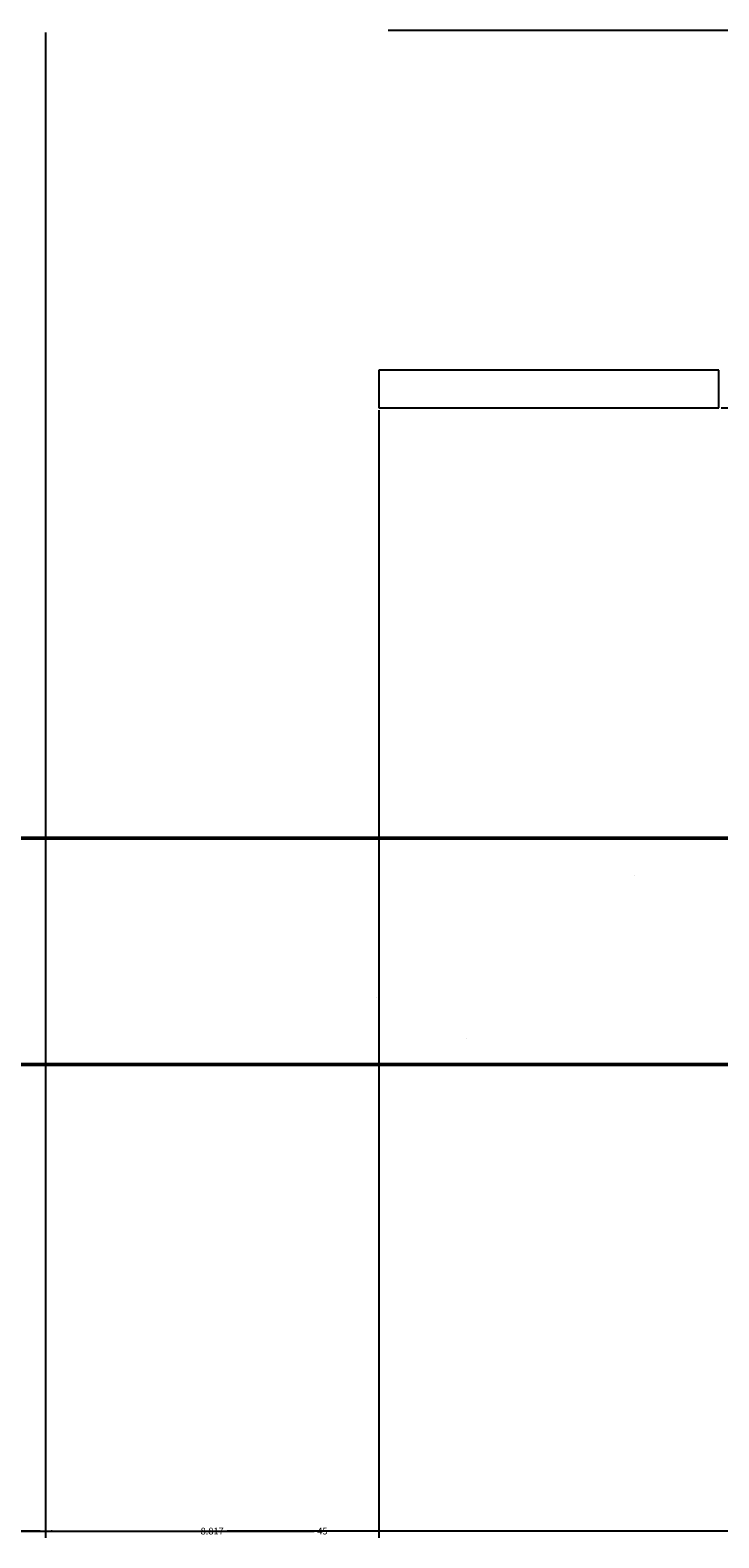
# Model space of a CAD drawing. Units: inches. Extents: x 2812 to 3051, y 1398 to 1659.
# Tile 15 of 65: x 2911 to 2929, y 1398 to 1437. Entities that reach past the tile are written whole.
import ezdxf

# ---------------------------------------------------------------- set-up
doc = ezdxf.new("R2010")
doc.units = ezdxf.units.IN
for name, color, linetype, lineweight in [('A-ANNO-DIMS', 2, 'Continuous', 18), ('S-CONC', 7, 'Continuous', 50), ('S-CONC-PATT', 8, 'Continuous', 18), ('S-STEP', 3, 'Continuous', 25)]:
    doc.layers.add(name, color=color, linetype=linetype, lineweight=lineweight)
doc.styles.get("Standard").update_dxf_attribs({"font": 'arial.ttf'})
doc.dimstyles.get("Standard").update_dxf_attribs({"dimtxt": 0.18, "dimasz": 0.18, "dimexe": 0.18, "dimexo": 0.0625, "dimgap": 0.09, "dimtad": 0, "dimtih": 1, "dimtoh": 1, "dimdec": 4, "dimzin": 0, "dimdsep": 46, "dimtxsty": 'Standard', "dimcen": 0.09, "dimadec": 0, "dimazin": 0, "dimtfac": 1, "dimtdec": 4, "dimtofl": 0, "dimtmove": 0, "dimatfit": 3, "dimfxl": 1, "dimtolj": 1, "dimtzin": 0, "dimarcsym": 0})

# ---------------------------------------------------------------- blocks, each defined once
blk = doc.blocks.new('STEP-IRON-3')
for p, q in [((9, 1), (0, 1)), ((0, 1), (0, 0)), ((9, 0), (9, 1)), ((0, 0), (4.457, 0)), ((0, 0), (9, 0)), ((0, 0), (5.792, 0))]:
    blk.add_line(p, q)
blk = doc.blocks.new('*D45')
at = {"layer": 'A-ANNO-DIMS', "color": 0, "lineweight": -2, "transparency": 16777216}
for p, q in [((2896.385, 1487.973), (2896.385, 1397.505)), ((2941.385, 1487.973), (2941.385, 1397.505)), ((2896.565, 1397.685), (2918.662, 1397.685)), ((2941.205, 1397.685), (2919.108, 1397.685))]:
    blk.add_line(p, q, dxfattribs=at)
at = {"layer": 'A-ANNO-DIMS', "color": 0, "transparency": 16777216}
for points in [[(2896.565, 1397.715), (2896.565, 1397.655), (2896.385, 1397.685)], [(2941.205, 1397.715), (2941.205, 1397.655), (2941.385, 1397.685)]]:
    blk.add_solid(points, dxfattribs=at)
at = {"layer": 'Defpoints', "color": 0, "transparency": 16777216}
for p in [(2896.385, 1488.035), (2941.385, 1488.035), (2941.385, 1397.685)]:
    blk.add_point(p, dxfattribs=at)
at = {"layer": 'A-ANNO-DIMS', "color": 0, "transparency": 16777216, "insert": (2918.885, 1397.685), "char_height": 0.18, "attachment_point": 5}
blk.add_mtext('\\A1;45', dxfattribs=at)
blk = doc.blocks.new('*D56')
at = {"layer": 'A-ANNO-DIMS', "color": 0, "lineweight": -2, "transparency": 16777216}
for p, q in [((2880.322, 1452.035), (2811.806, 1452.035)), ((2811.986, 1451.855), (2811.986, 1434.217)), ((2811.986, 1416.215), (2811.986, 1433.853)), ((2952.322, 1416.035), (2811.806, 1416.035))]:
    blk.add_line(p, q, dxfattribs=at)
at = {"layer": 'A-ANNO-DIMS', "color": 0, "transparency": 16777216}
for points in [[(2811.956, 1451.855), (2812.016, 1451.855), (2811.986, 1452.035)], [(2811.956, 1416.215), (2812.016, 1416.215), (2811.986, 1416.035)]]:
    blk.add_solid(points, dxfattribs=at)
at = {"layer": 'Defpoints', "color": 0, "transparency": 16777216}
for p in [(2811.986, 1452.035), (2880.385, 1452.035), (2952.385, 1416.035)]:
    blk.add_point(p, dxfattribs=at)
at = {"layer": 'A-ANNO-DIMS', "color": 0, "transparency": 16777216, "insert": (2811.986, 1434.035), "char_height": 0.18, "attachment_point": 5}
blk.add_mtext('\\A1;36', dxfattribs=at)
blk = doc.blocks.new('*D62')
at = {"layer": 'A-ANNO-DIMS', "color": 0, "lineweight": -2, "transparency": 16777216}
for p, q in [((2904.955, 1447.364), (2904.955, 1397.505)), ((2911.558, 1437.364), (2911.558, 1397.505)), ((2905.135, 1397.685), (2907.862, 1397.685)), ((2911.378, 1397.685), (2908.651, 1397.685))]:
    blk.add_line(p, q, dxfattribs=at)
at = {"layer": 'A-ANNO-DIMS', "color": 0, "transparency": 16777216}
for points in [[(2905.135, 1397.715), (2905.135, 1397.655), (2904.955, 1397.685)], [(2911.378, 1397.715), (2911.378, 1397.655), (2911.558, 1397.685)]]:
    blk.add_solid(points, dxfattribs=at)
at = {"layer": 'Defpoints', "color": 0, "transparency": 16777216}
for p in [(2904.955, 1447.426), (2911.558, 1437.426), (2911.558, 1397.685)]:
    blk.add_point(p, dxfattribs=at)
at = {"layer": 'A-ANNO-DIMS', "color": 0, "transparency": 16777216, "insert": (2908.256, 1397.685), "char_height": 0.18, "attachment_point": 5}
blk.add_mtext('\\A1;6.603', dxfattribs=at)
blk = doc.blocks.new('*D63')
at = {"layer": 'A-ANNO-DIMS', "color": 0, "lineweight": -2, "transparency": 16777216}
for p, q in [((2911.558, 1437.364), (2911.558, 1397.505)), ((2920.375, 1427.364), (2920.375, 1397.505)), ((2911.738, 1397.685), (2915.573, 1397.685)), ((2920.195, 1397.685), (2916.36, 1397.685))]:
    blk.add_line(p, q, dxfattribs=at)
at = {"layer": 'A-ANNO-DIMS', "color": 0, "transparency": 16777216}
for points in [[(2911.738, 1397.715), (2911.738, 1397.655), (2911.558, 1397.685)], [(2920.195, 1397.715), (2920.195, 1397.655), (2920.375, 1397.685)]]:
    blk.add_solid(points, dxfattribs=at)
at = {"layer": 'Defpoints', "color": 0, "transparency": 16777216}
for p in [(2911.558, 1437.426), (2920.375, 1427.426), (2920.375, 1397.685)]:
    blk.add_point(p, dxfattribs=at)
at = {"layer": 'A-ANNO-DIMS', "color": 0, "transparency": 16777216, "insert": (2915.966, 1397.685), "char_height": 0.18, "attachment_point": 5}
blk.add_mtext('\\A1;8.817', dxfattribs=at)
blk = doc.blocks.new('*D65')
at = {"layer": 'A-ANNO-DIMS', "color": 0, "lineweight": -2, "transparency": 16777216}
for p, q in [((2920.62, 1437.426), (3051.178, 1437.426)), ((3050.998, 1437.246), (3050.998, 1432.608)), ((3050.998, 1427.606), (3050.998, 1432.245)), ((2929.438, 1427.426), (3051.178, 1427.426))]:
    blk.add_line(p, q, dxfattribs=at)
at = {"layer": 'A-ANNO-DIMS', "color": 0, "transparency": 16777216}
for points in [[(3050.968, 1437.246), (3051.028, 1437.246), (3050.998, 1437.426)], [(3050.968, 1427.606), (3051.028, 1427.606), (3050.998, 1427.426)]]:
    blk.add_solid(points, dxfattribs=at)
at = {"layer": 'Defpoints', "color": 0, "transparency": 16777216}
for p in [(2920.558, 1437.426), (3050.998, 1437.426), (2929.375, 1427.426)]:
    blk.add_point(p, dxfattribs=at)
at = {"layer": 'A-ANNO-DIMS', "color": 0, "transparency": 16777216, "insert": (3050.998, 1432.426), "char_height": 0.18, "attachment_point": 5}
blk.add_mtext('\\A1;10', dxfattribs=at)
blk = doc.blocks.new('*D66')
at = {"layer": 'A-ANNO-DIMS', "color": 0, "lineweight": -2, "transparency": 16777216}
for p, q in [((2914.018, 1447.426), (3051.178, 1447.426)), ((3050.998, 1447.246), (3050.998, 1442.608)), ((3050.998, 1437.606), (3050.998, 1442.245)), ((2920.62, 1437.426), (3051.178, 1437.426))]:
    blk.add_line(p, q, dxfattribs=at)
at = {"layer": 'A-ANNO-DIMS', "color": 0, "transparency": 16777216}
for points in [[(3050.968, 1447.246), (3051.028, 1447.246), (3050.998, 1447.426)], [(3050.968, 1437.606), (3051.028, 1437.606), (3050.998, 1437.426)]]:
    blk.add_solid(points, dxfattribs=at)
at = {"layer": 'Defpoints', "color": 0, "transparency": 16777216}
for p in [(2913.955, 1447.426), (3050.998, 1447.426), (2920.558, 1437.426)]:
    blk.add_point(p, dxfattribs=at)
at = {"layer": 'A-ANNO-DIMS', "color": 0, "transparency": 16777216, "insert": (3050.998, 1442.426), "char_height": 0.18, "attachment_point": 5}
blk.add_mtext('\\A1;10', dxfattribs=at)
blk = doc.blocks.new('*D75')
at = {"layer": 'A-ANNO-DIMS', "color": 0, "lineweight": -2, "transparency": 16777216}
for p, q in [((2963.812, 1448.474), (2811.806, 1448.474)), ((2811.986, 1448.294), (2811.986, 1432.437)), ((2811.986, 1416.215), (2811.986, 1432.073)), ((2961.322, 1416.035), (2811.806, 1416.035))]:
    blk.add_line(p, q, dxfattribs=at)
at = {"layer": 'A-ANNO-DIMS', "color": 0, "transparency": 16777216}
for points in [[(2811.956, 1448.294), (2812.016, 1448.294), (2811.986, 1448.474)], [(2811.956, 1416.215), (2812.016, 1416.215), (2811.986, 1416.035)]]:
    blk.add_solid(points, dxfattribs=at)
at = {"layer": 'Defpoints', "color": 0, "transparency": 16777216}
for p in [(2811.986, 1448.474), (2963.874, 1448.474), (2961.385, 1416.035)]:
    blk.add_point(p, dxfattribs=at)
at = {"layer": 'A-ANNO-DIMS', "color": 0, "transparency": 16777216, "insert": (2811.986, 1432.255), "char_height": 0.18, "attachment_point": 5}
blk.add_mtext('\\A1;32.44', dxfattribs=at)

msp = doc.modelspace()

# ---------------------------------------------------------------- hatches: boundary and pattern name
at = {"layer": 'S-CONC-PATT'}
h = msp.add_hatch(dxfattribs=at)
h.set_pattern_fill('AR-SAND', color=256, scale=0.3)
h.paths.add_polyline_path([(3036.3849, 1416.0354), (3027.3849, 1416.0354), (2826.3849, 1416.0354), (2826.3849, 1410.0354), (2835.3849, 1410.0354), (3036.3849, 1410.0354)])
h.paths.add_polyline_path([(2970.3849, 1488.0354), (2969.3849, 1488.0354), (2941.3849, 1488.0354), (2941.3849, 1482.0354), (2970.3849, 1482.0354)])
h.paths.add_polyline_path([(3036.3849, 1488.0354), (3035.3849, 1488.0354), (3006.3849, 1488.0354), (3006.3849, 1482.0354), (3027.3849, 1482.0354), (3036.3849, 1482.0354)])
h.paths.add_polyline_path([(3034.3849, 1490.0354), (3008.3849, 1490.0354), (3008.3849, 1489.0354), (3034.3849, 1489.0354)])
h.paths.add_polyline_path([(3035.3849, 1489.0354), (3034.3849, 1489.0354), (3007.3849, 1489.0354), (3007.3849, 1488.0354), (3035.3849, 1488.0354)])
h.paths.add_polyline_path([(2968.3849, 1490.0354), (2943.3849, 1490.0354), (2943.3849, 1489.0354), (2968.3849, 1489.0354)])
h.paths.add_polyline_path([(2969.3849, 1489.0354), (2968.3849, 1489.0354), (2942.3849, 1489.0354), (2942.3849, 1488.0354), (2969.3849, 1488.0354)])
h.paths.add_polyline_path([(2896.3849, 1488.0354), (2826.3849, 1488.0354), (2826.3849, 1482.0354), (2896.3849, 1482.0354)])
h.paths.add_polyline_path([(2895.3849, 1489.0354), (2894.3849, 1489.0354), (2827.3849, 1489.0354), (2827.3849, 1488.0354), (2895.3849, 1488.0354)])
h.paths.add_polyline_path([(2894.3849, 1490.0354), (2828.3849, 1490.0354), (2828.3849, 1489.0354), (2894.3849, 1489.0354)])
h = msp.add_hatch(dxfattribs=at)
h.set_pattern_fill('AR-CONC', color=256, scale=0.3)
h.paths.add_polyline_path([(3036.3849, 1416.0354), (3027.3849, 1416.0354), (2826.3849, 1416.0354), (2826.3849, 1410.0354), (2835.3849, 1410.0354), (3036.3849, 1410.0354)])

# ---------------------------------------------------------------- linework, layer by layer
at = {"layer": 'S-CONC'}
for p, q in [((2826.3849, 1416.0354), (3027.3849, 1416.0354)), ((2835.3849, 1410.0354), (3036.3849, 1410.0354))]:
    msp.add_line(p, q, dxfattribs=at)

# ---------------------------------------------------------------- block references
at = {"layer": 'S-STEP'}
msp.add_blockref('STEP-IRON-3', (2920.3754, 1427.4261), dxfattribs=at)

# ---------------------------------------------------------------- dimensions: what is measured, and where the dimension line sits
at = {"layer": 'A-ANNO-DIMS'}
for base, p1, p2, override, picture, middle in [((2941.3849, 1397.6854), (2896.3849, 1488.0354), (2941.3849, 1488.0354), {"dimdec": 0, "dimlfac": 1, "dimrnd": 0, "dimzin": 0, "dimdsep": 46, "dimlunit": 2}, '*D45', (2918.8849, 1397.6854)), ((2911.5577, 1397.6854), (2904.9551, 1447.4265), (2911.5577, 1437.4265), {"dimdec": 3, "dimlfac": 1, "dimrnd": 0, "dimzin": 0, "dimdsep": 46, "dimlunit": 2}, '*D62', (2908.2564, 1397.6854)), ((2920.3751, 1397.6854), (2911.5577, 1437.4265), (2920.3751, 1427.4265), {"dimdec": 3, "dimlfac": 1, "dimrnd": 0, "dimzin": 0, "dimdsep": 46, "dimlunit": 2}, '*D63', (2915.9664, 1397.6854))]:
    dim = msp.add_linear_dim(base=base, p1=p1, p2=p2, dimstyle='Standard', override=override, dxfattribs=at)
    dim.commit()
    dim.dimension.update_dxf_attribs({"geometry": picture, "text_midpoint": middle})
for base, p1, p2, override, picture, middle in [((2811.9855, 1452.0354), (2952.3849, 1416.0354), (2880.3849, 1452.0354), {"dimdec": 0, "dimlfac": 1, "dimrnd": 0, "dimzin": 0, "dimdsep": 46, "dimlunit": 2}, '*D56', (2811.9855, 1434.0354)), ((2811.9855, 1448.4738), (2961.3849, 1416.0354), (2963.8741, 1448.4738), {"dimdec": 2, "dimlfac": 1, "dimrnd": 0, "dimzin": 0, "dimdsep": 46, "dimlunit": 2}, '*D75', (2811.9855, 1432.2546)), ((3050.998, 1447.4265), (2920.5577, 1437.4265), (2913.9551, 1447.4265), {"dimdec": 0, "dimlfac": 1, "dimrnd": 0, "dimzin": 0, "dimdsep": 46, "dimlunit": 2}, '*D66', (3050.998, 1442.4265)), ((3050.998, 1437.4265), (2929.3751, 1427.4265), (2920.5577, 1437.4265), {"dimdec": 0, "dimlfac": 1, "dimrnd": 0, "dimzin": 0, "dimdsep": 46, "dimlunit": 2}, '*D65', (3050.998, 1432.4265))]:
    dim = msp.add_linear_dim(base=base, p1=p1, p2=p2, angle=90, dimstyle='Standard', override=override, dxfattribs=at)
    dim.commit()
    dim.dimension.update_dxf_attribs({"geometry": picture, "text_midpoint": middle})

doc.saveas('drawing.dxf')
